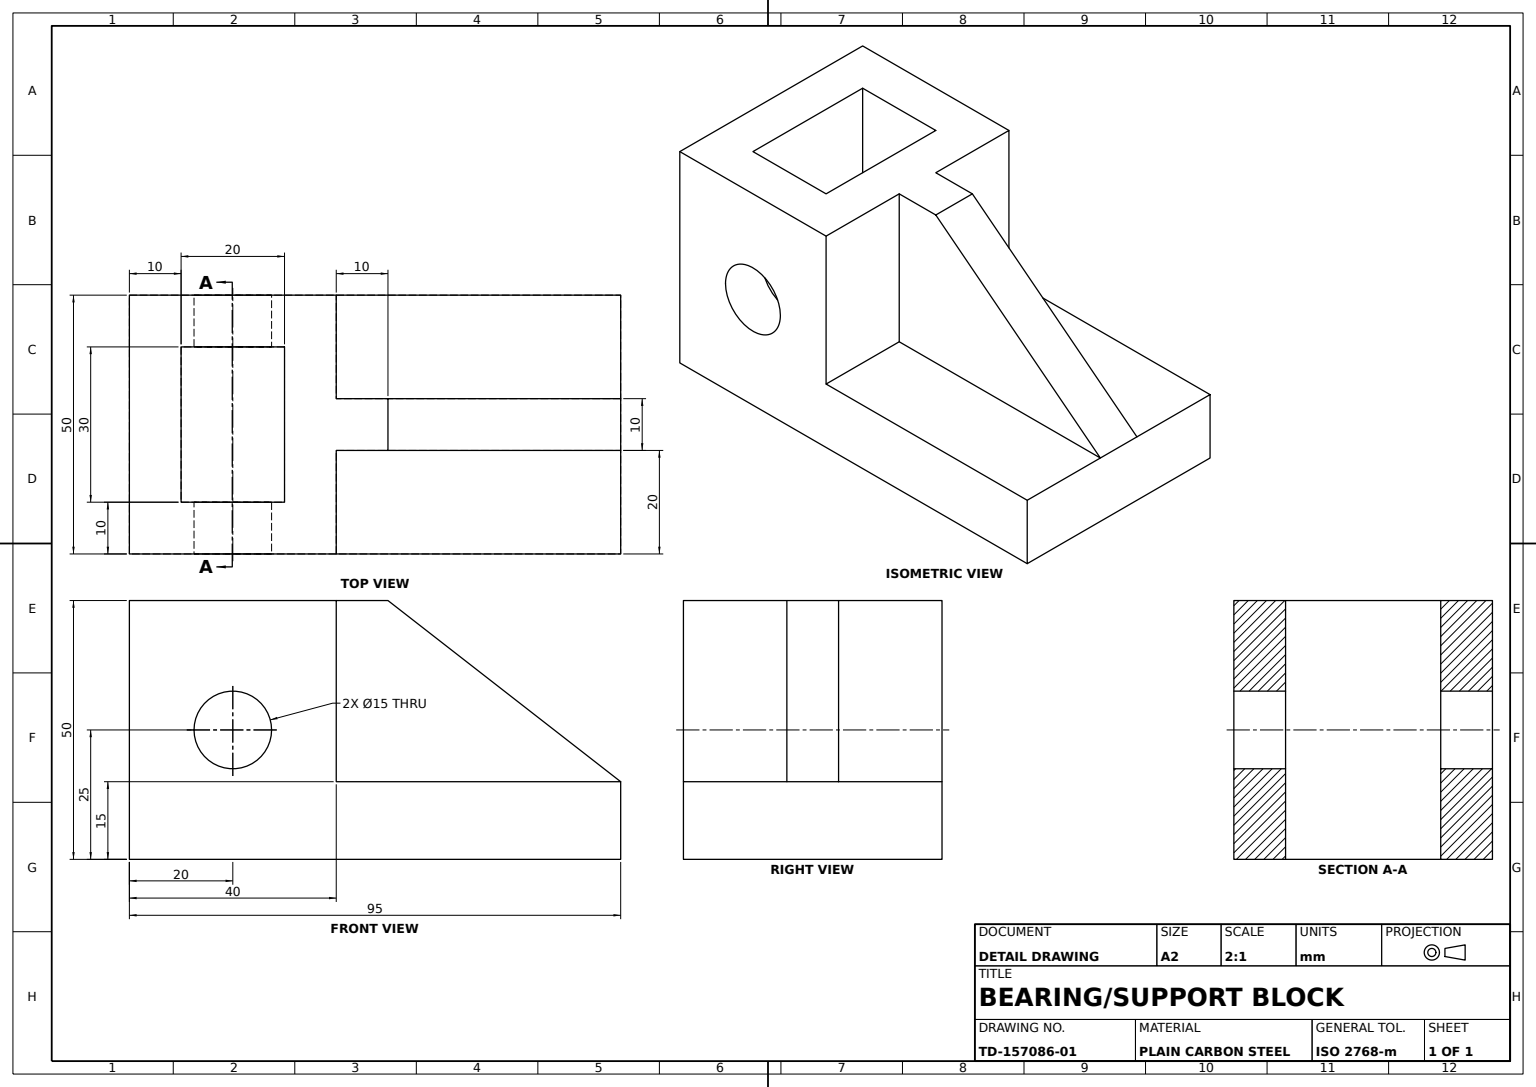
SolidWorks part; units mm, degrees
material "Plain Carbon Steel"
ref_plane "Front Plane" through (0, 0, 0) normal (0, 0, 1) x (1, 0, 0)
ref_plane "Top Plane" through (0, 0, 0) normal (0, 1, 0) x (1, 0, 0)
ref_plane "Right Plane" through (0, 0, 0) normal (1, 0, 0) x (0, 0, -1)
sketch "Bracket Profile Sketch" plane through (0, 0, 0) normal (0, 0, 1) x (1, 0, 0)
  line L0 (0, 0) -> (95, 0)
  line L1 (95, 0) -> (95, 15)
  line L2 (0, 0) -> (0, 50)
  line L3 (0, 50) -> (40, 50)
  line L4 (40, 50) -> (40, 15)
  line L5 (40, 15) -> (95, 15)
  dimension "D1" = 40
  dimension "D2" = 95
  dimension "D3" = 15
  dimension "D4" = 50
extrude "Bracket Base 50mm" add sketch "Bracket Profile Sketch" along normal blind 50
sketch "Hole 1 Sketch" plane through (0, 0, 50) normal (0, 0, 1) x (1, 0, 0)
  line L0 (0, 50) -> (0, 0) construction
  line L1 (0, 0) -> (95, 0) construction
  circle A0 centre (20, 25) radius 7.5
  dimension "D1" = 15
  dimension "D2" = 20
  dimension "D3" = 25
extrude "Hole 1 Cut 10mm Deep" cut sketch "Hole 1 Sketch" against normal blind 10
sketch "Hole 2 Sketch" plane through (0, 0, 0) normal (0, 0, -1) x (-1, 0, 0)
  line L0 (0, 50) -> (0, 0) construction
  line L1 (-40, 50) -> (0, 50) construction
  circle A0 centre (-20, 25) radius 7.5
  dimension "D1" = 15
  dimension "D2" = 20
  dimension "D3" = 25
extrude "Hole 2 Cut 10mm Deep" cut sketch "Hole 2 Sketch" against normal blind 10
sketch "Raised Boss Sketch" plane through (0, 50, 0) normal (0, 1, 0) x (1, 0, 0)
  line L1 (50, -20) -> (40, -20)
  line L2 (50, -20) -> (50, -30)
  line L3 (50, -30) -> (40, -30)
  line L4 (40, -20) -> (40, -30)
  line L5 (50, -20) -> (40, -30) construction
  line L6 (50, -30) -> (40, -20) construction
  line L7 (40, -50) -> (40, 0) construction
  line L8 (40, 0) -> (0, 0) construction
  point P0 (40, -25)
  dimension "D1" = 10
  dimension "D2" = 20
extrude "Raised Boss 35mm" add sketch "Raised Boss Sketch" against normal blind 35
ref_plane "Rib Mid Plane" through (0, 0, 25) normal (0, 0, 1) x (1, 0, 0)
sketch "Gusset Rib Sketch" plane through (0, 0, 25) normal (0, 0, 1) x (1, 0, 0)
  line L0 (50, 50) -> (95, 15)
rib "Gusset Rib 10mm" sketch "Gusset Rib Sketch" sketch "Gusset Rib Sketch" thickness 10 extrusion direction parallel to sketch draft on no parameters "D1"=10
sketch "Square Pocket Sketch" plane through (0, 50, 0) normal (0, 1, 0) x (1, 0, 0)
  line L0 (40, 0) -> (0, 0) construction
  line L1 (10, -10) -> (30, -10)
  line L2 (10, -10) -> (10, -40)
  line L3 (10, -40) -> (30, -40)
  line L4 (30, -10) -> (30, -40)
  line L5 (10, -10) -> (30, -40) construction
  line L6 (10, -40) -> (30, -10) construction
  line L7 (0, -50) -> (0, 0) construction
  point P0 (20, -25)
  dimension "D1" = 10
  dimension "D2" = 10
  dimension "D3" = 20
  dimension "D4" = 30
extrude "Square Pocket Cut" cut sketch "Square Pocket Sketch" against normal through all
